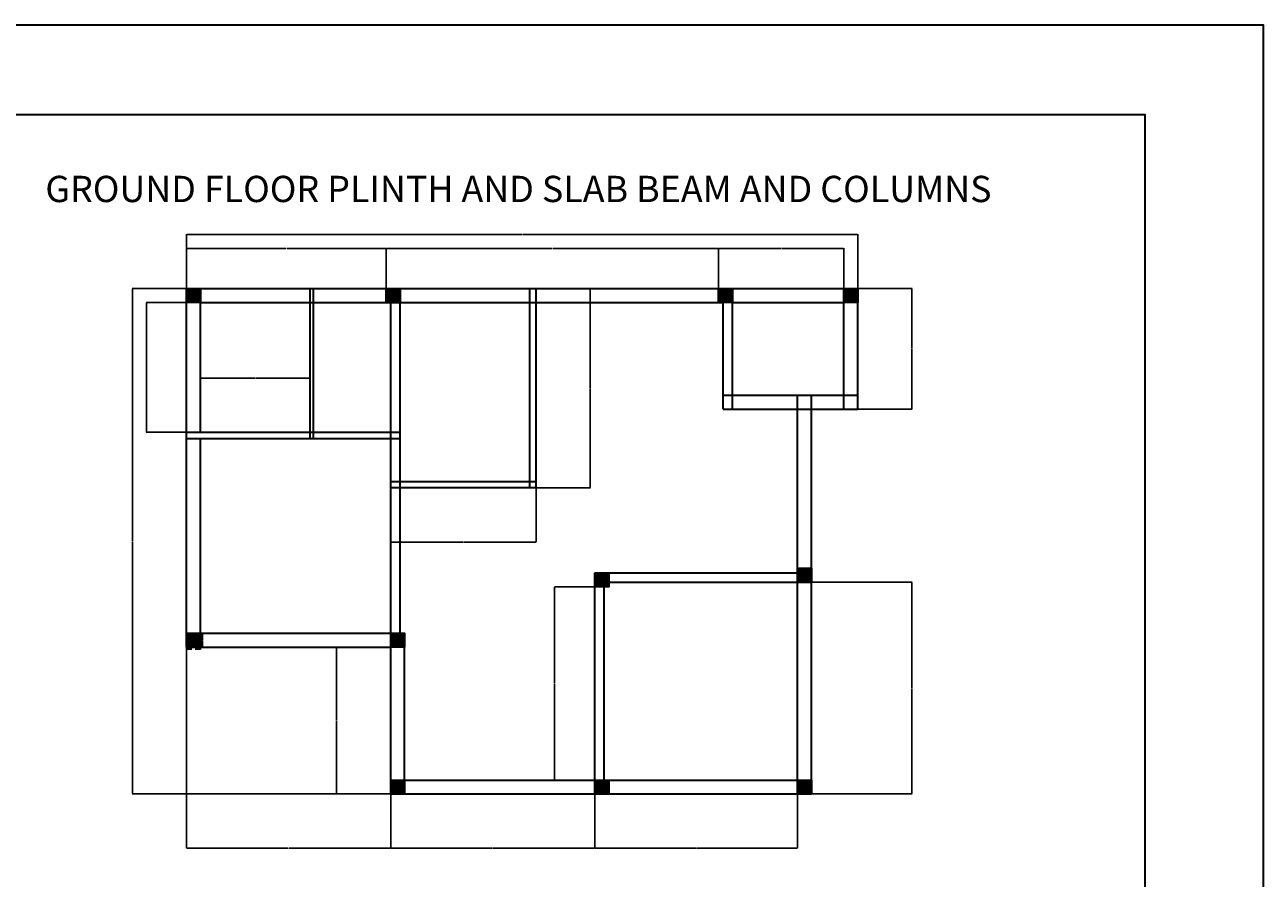
# Model space of a CAD drawing. Units: inches. Extents: x 2286 to 3750, y 1240 to 2345.
# Tile 7 of 7: x 2949 to 3750, y 1793 to 2345. Entities that reach past the tile are written whole.
import ezdxf

# ---------------------------------------------------------------- set-up
doc = ezdxf.new("R2010")
doc.units = ezdxf.units.IN
for name, color, linetype, lineweight in [('A-ANNO-DIMS', 2, 'Continuous', 18), ('A-ANNO-TEXT', 7, 'Continuous', 35), ('A-WALL', 7, 'Continuous', 35), ('S-BEAM', 7, 'Continuous', 30), ('S-COLS', 1, 'Continuous', 35)]:
    doc.layers.add(name, color=color, linetype=linetype, lineweight=lineweight)
doc.styles.get("Standard").update_dxf_attribs({"font": 'arial.ttf'})
doc.dimstyles.get("Standard").update_dxf_attribs({"dimtxt": 0.18, "dimasz": 0.18, "dimexe": 0.18, "dimexo": 0.0625, "dimgap": 0.09, "dimtad": 0, "dimtih": 1, "dimtoh": 1, "dimdec": 4, "dimzin": 0, "dimdsep": 46, "dimtxsty": 'Standard', "dimcen": 0.09, "dimadec": 0, "dimazin": 0, "dimtfac": 1, "dimtdec": 4, "dimtofl": 0, "dimtmove": 0, "dimatfit": 3, "dimfxl": 1, "dimtolj": 1, "dimtzin": 0, "dimarcsym": 0})

# ---------------------------------------------------------------- blocks, each defined once
blk = doc.blocks.new('COL-9-SQ')
h = blk.add_hatch(color=256)
h.dxf.hatch_style = 1
h.paths.add_polyline_path([(0, 0), (9, 0), (9, 9), (0, 9)])
blk.add_lwpolyline([(0, 9), (9, 9), (9, 0), (0, 0)], close=True)
blk = doc.blocks.new('*D22')
at = {"layer": 'A-ANNO-DIMS', "color": 0, "lineweight": -2, "transparency": 16777216}
for p, q in [((3054.05, 1942.13), (3054.05, 1940.66)), ((3054.23, 1940.84), (3057.51, 1940.84)), ((3062.87, 1940.84), (3059.59, 1940.84)), ((3063.05, 1942.13), (3063.05, 1940.66))]:
    blk.add_line(p, q, dxfattribs=at)
at = {"layer": 'A-ANNO-DIMS', "color": 0, "transparency": 16777216}
for points in [[(3054.23, 1940.87), (3054.23, 1940.81), (3054.05, 1940.84)], [(3062.87, 1940.87), (3062.87, 1940.81), (3063.05, 1940.84)]]:
    blk.add_solid(points, dxfattribs=at)
at = {"layer": 'Defpoints', "color": 0, "transparency": 16777216}
for p in [(3054.05, 1942.19), (3063.05, 1942.19), (3063.05, 1940.84)]:
    blk.add_point(p, dxfattribs=at)
at = {"layer": 'A-ANNO-DIMS', "color": 0, "transparency": 16777216, "insert": (3058.55, 1940.84), "char_height": 0.18, "attachment_point": 5}
blk.add_mtext('\\A1;COLUMN 9 TYP.', dxfattribs=at)
blk = doc.blocks.new('*D23')
at = {"layer": 'A-ANNO-DIMS', "color": 0, "lineweight": -2, "transparency": 16777216}
for p, q in [((3063.11, 1951.19), (3064.58, 1951.19)), ((3064.4, 1951.01), (3064.4, 1946.87)), ((3064.4, 1942.37), (3064.4, 1946.51)), ((3063.11, 1942.19), (3064.58, 1942.19))]:
    blk.add_line(p, q, dxfattribs=at)
at = {"layer": 'A-ANNO-DIMS', "color": 0, "transparency": 16777216}
for points in [[(3064.37, 1951.01), (3064.43, 1951.01), (3064.4, 1951.19)], [(3064.37, 1942.37), (3064.43, 1942.37), (3064.4, 1942.19)]]:
    blk.add_solid(points, dxfattribs=at)
at = {"layer": 'Defpoints', "color": 0, "transparency": 16777216}
for p in [(3063.05, 1951.19), (3064.4, 1951.19), (3063.05, 1942.19)]:
    blk.add_point(p, dxfattribs=at)
at = {"layer": 'A-ANNO-DIMS', "color": 0, "transparency": 16777216, "insert": (3064.4, 1946.69), "char_height": 0.18, "attachment_point": 5}
blk.add_mtext('\\A1;9 TYP.', dxfattribs=at)
blk = doc.blocks.new('*D93')
at = {"layer": 'A-ANNO-DIMS', "color": 0, "lineweight": -2, "transparency": 16777216}
for p, q in [((3054.05, 2174.25), (3054.05, 2209.37)), ((3054.23, 2209.19), (3270.76, 2209.19)), ((3487.87, 2209.19), (3271.34, 2209.19)), ((3488.05, 2174.25), (3488.05, 2209.37))]:
    blk.add_line(p, q, dxfattribs=at)
at = {"layer": 'A-ANNO-DIMS', "color": 0, "transparency": 16777216}
for points in [[(3054.23, 2209.22), (3054.23, 2209.16), (3054.05, 2209.19)], [(3487.87, 2209.22), (3487.87, 2209.16), (3488.05, 2209.19)]]:
    blk.add_solid(points, dxfattribs=at)
at = {"layer": 'Defpoints', "color": 0, "transparency": 16777216}
for p in [(3488.05, 2209.19), (3054.05, 2174.19), (3488.05, 2174.19)]:
    blk.add_point(p, dxfattribs=at)
at = {"layer": 'A-ANNO-DIMS', "color": 0, "transparency": 16777216, "insert": (3271.05, 2209.19), "char_height": 0.18, "attachment_point": 5}
blk.add_mtext('\\A1;434', dxfattribs=at)
blk = doc.blocks.new('*D94')
at = {"layer": 'A-ANNO-DIMS', "color": 0, "lineweight": -2, "transparency": 16777216}
for p, q in [((3053.99, 2174.19), (3018.87, 2174.19)), ((3019.05, 2174.01), (3019.05, 2010.87)), ((3019.05, 1847.37), (3019.05, 2010.51)), ((3185.99, 1847.19), (3018.87, 1847.19))]:
    blk.add_line(p, q, dxfattribs=at)
at = {"layer": 'A-ANNO-DIMS', "color": 0, "transparency": 16777216}
for points in [[(3019.02, 2174.01), (3019.08, 2174.01), (3019.05, 2174.19)], [(3019.02, 1847.37), (3019.08, 1847.37), (3019.05, 1847.19)]]:
    blk.add_solid(points, dxfattribs=at)
at = {"layer": 'Defpoints', "color": 0, "transparency": 16777216}
for p in [(3054.05, 2174.19), (3019.05, 1847.19), (3186.05, 1847.19)]:
    blk.add_point(p, dxfattribs=at)
at = {"layer": 'A-ANNO-DIMS', "color": 0, "transparency": 16777216, "insert": (3019.05, 2010.69), "char_height": 0.18, "attachment_point": 5}
blk.add_mtext('\\A1;327', dxfattribs=at)
blk = doc.blocks.new('*D95')
at = {"layer": 'A-ANNO-DIMS', "color": 0, "lineweight": -2, "transparency": 16777216}
for p, q in [((3054.05, 2165.25), (3054.05, 2200.37)), ((3054.23, 2200.19), (3118.27, 2200.19)), ((3182.87, 2200.19), (3118.83, 2200.19)), ((3183.05, 2165.25), (3183.05, 2200.37))]:
    blk.add_line(p, q, dxfattribs=at)
at = {"layer": 'A-ANNO-DIMS', "color": 0, "transparency": 16777216}
for points in [[(3054.23, 2200.22), (3054.23, 2200.16), (3054.05, 2200.19)], [(3182.87, 2200.22), (3182.87, 2200.16), (3183.05, 2200.19)]]:
    blk.add_solid(points, dxfattribs=at)
at = {"layer": 'Defpoints', "color": 0, "transparency": 16777216}
for p in [(3183.05, 2200.19), (3054.05, 2165.19), (3183.05, 2165.19)]:
    blk.add_point(p, dxfattribs=at)
at = {"layer": 'A-ANNO-DIMS', "color": 0, "transparency": 16777216, "insert": (3118.55, 2200.19), "char_height": 0.18, "attachment_point": 5}
blk.add_mtext('\\A1;129', dxfattribs=at)
blk = doc.blocks.new('*D96')
at = {"layer": 'A-ANNO-DIMS', "color": 0, "lineweight": -2, "transparency": 16777216}
for p, q in [((3183.05, 2165.25), (3183.05, 2200.37)), ((3183.23, 2200.19), (3290.26, 2200.19)), ((3397.87, 2200.19), (3290.84, 2200.19)), ((3398.05, 2165.25), (3398.05, 2200.37))]:
    blk.add_line(p, q, dxfattribs=at)
at = {"layer": 'A-ANNO-DIMS', "color": 0, "transparency": 16777216}
for points in [[(3183.23, 2200.22), (3183.23, 2200.16), (3183.05, 2200.19)], [(3397.87, 2200.22), (3397.87, 2200.16), (3398.05, 2200.19)]]:
    blk.add_solid(points, dxfattribs=at)
at = {"layer": 'Defpoints', "color": 0, "transparency": 16777216}
for p in [(3398.05, 2200.19), (3183.05, 2165.19), (3398.05, 2165.19)]:
    blk.add_point(p, dxfattribs=at)
at = {"layer": 'A-ANNO-DIMS', "color": 0, "transparency": 16777216, "insert": (3290.55, 2200.19), "char_height": 0.18, "attachment_point": 5}
blk.add_mtext('\\A1;215', dxfattribs=at)
blk = doc.blocks.new('*D97')
at = {"layer": 'A-ANNO-DIMS', "color": 0, "lineweight": -2, "transparency": 16777216}
for p, q in [((3398.05, 2165.25), (3398.05, 2200.37)), ((3398.23, 2200.19), (3438.35, 2200.19)), ((3478.87, 2200.19), (3438.75, 2200.19)), ((3479.05, 2165.25), (3479.05, 2200.37))]:
    blk.add_line(p, q, dxfattribs=at)
at = {"layer": 'A-ANNO-DIMS', "color": 0, "transparency": 16777216}
for points in [[(3398.23, 2200.22), (3398.23, 2200.16), (3398.05, 2200.19)], [(3478.87, 2200.22), (3478.87, 2200.16), (3479.05, 2200.19)]]:
    blk.add_solid(points, dxfattribs=at)
at = {"layer": 'Defpoints', "color": 0, "transparency": 16777216}
for p in [(3479.05, 2200.19), (3398.05, 2165.19), (3479.05, 2165.19)]:
    blk.add_point(p, dxfattribs=at)
at = {"layer": 'A-ANNO-DIMS', "color": 0, "transparency": 16777216, "insert": (3438.55, 2200.19), "char_height": 0.18, "attachment_point": 5}
blk.add_mtext('\\A1;81', dxfattribs=at)
blk = doc.blocks.new('*D98')
at = {"layer": 'A-ANNO-DIMS', "color": 0, "lineweight": -2, "transparency": 16777216}
for p, q in [((3054.05, 1942.13), (3054.05, 1812.01)), ((3186.05, 1942.13), (3186.05, 1812.01)), ((3054.23, 1812.19), (3119.77, 1812.19)), ((3185.87, 1812.19), (3120.33, 1812.19))]:
    blk.add_line(p, q, dxfattribs=at)
at = {"layer": 'A-ANNO-DIMS', "color": 0, "transparency": 16777216}
for points in [[(3054.23, 1812.22), (3054.23, 1812.16), (3054.05, 1812.19)], [(3185.87, 1812.22), (3185.87, 1812.16), (3186.05, 1812.19)]]:
    blk.add_solid(points, dxfattribs=at)
at = {"layer": 'Defpoints', "color": 0, "transparency": 16777216}
for p in [(3054.05, 1942.19), (3186.05, 1942.19), (3186.05, 1812.19)]:
    blk.add_point(p, dxfattribs=at)
at = {"layer": 'A-ANNO-DIMS', "color": 0, "transparency": 16777216, "insert": (3120.05, 1812.19), "char_height": 0.18, "attachment_point": 5}
blk.add_mtext('\\A1;132', dxfattribs=at)
blk = doc.blocks.new('*D99')
at = {"layer": 'A-ANNO-DIMS', "color": 0, "lineweight": -2, "transparency": 16777216}
for p, q in [((3186.05, 1847.13), (3186.05, 1812.01)), ((3318.05, 1847.13), (3318.05, 1812.01)), ((3186.23, 1812.19), (3251.77, 1812.19)), ((3317.87, 1812.19), (3252.33, 1812.19))]:
    blk.add_line(p, q, dxfattribs=at)
at = {"layer": 'A-ANNO-DIMS', "color": 0, "transparency": 16777216}
for points in [[(3186.23, 1812.22), (3186.23, 1812.16), (3186.05, 1812.19)], [(3317.87, 1812.22), (3317.87, 1812.16), (3318.05, 1812.19)]]:
    blk.add_solid(points, dxfattribs=at)
at = {"layer": 'Defpoints', "color": 0, "transparency": 16777216}
for p in [(3186.05, 1847.19), (3318.05, 1847.19), (3318.05, 1812.19)]:
    blk.add_point(p, dxfattribs=at)
at = {"layer": 'A-ANNO-DIMS', "color": 0, "transparency": 16777216, "insert": (3252.05, 1812.19), "char_height": 0.18, "attachment_point": 5}
blk.add_mtext('\\A1;132', dxfattribs=at)
blk = doc.blocks.new('*D100')
at = {"layer": 'A-ANNO-DIMS', "color": 0, "lineweight": -2, "transparency": 16777216}
for p, q in [((3318.05, 1847.13), (3318.05, 1812.01)), ((3449.05, 1847.13), (3449.05, 1812.01)), ((3318.23, 1812.19), (3383.29, 1812.19)), ((3448.87, 1812.19), (3383.81, 1812.19))]:
    blk.add_line(p, q, dxfattribs=at)
at = {"layer": 'A-ANNO-DIMS', "color": 0, "transparency": 16777216}
for points in [[(3318.23, 1812.22), (3318.23, 1812.16), (3318.05, 1812.19)], [(3448.87, 1812.22), (3448.87, 1812.16), (3449.05, 1812.19)]]:
    blk.add_solid(points, dxfattribs=at)
at = {"layer": 'Defpoints', "color": 0, "transparency": 16777216}
for p in [(3318.05, 1847.19), (3449.05, 1847.19), (3449.05, 1812.19)]:
    blk.add_point(p, dxfattribs=at)
at = {"layer": 'A-ANNO-DIMS', "color": 0, "transparency": 16777216, "insert": (3383.55, 1812.19), "char_height": 0.18, "attachment_point": 5}
blk.add_mtext('\\A1;131', dxfattribs=at)
blk = doc.blocks.new('*D101')
at = {"layer": 'A-ANNO-DIMS', "color": 0, "lineweight": -2, "transparency": 16777216}
for p, q in [((3185.99, 1942.19), (3150.87, 1942.19)), ((3151.05, 1942.01), (3151.05, 1894.87)), ((3151.05, 1847.37), (3151.05, 1894.51)), ((3185.99, 1847.19), (3150.87, 1847.19))]:
    blk.add_line(p, q, dxfattribs=at)
at = {"layer": 'A-ANNO-DIMS', "color": 0, "transparency": 16777216}
for points in [[(3151.02, 1942.01), (3151.08, 1942.01), (3151.05, 1942.19)], [(3151.02, 1847.37), (3151.08, 1847.37), (3151.05, 1847.19)]]:
    blk.add_solid(points, dxfattribs=at)
at = {"layer": 'Defpoints', "color": 0, "transparency": 16777216}
for p in [(3151.05, 1942.19), (3186.05, 1942.19), (3186.05, 1847.19)]:
    blk.add_point(p, dxfattribs=at)
at = {"layer": 'A-ANNO-DIMS', "color": 0, "transparency": 16777216, "insert": (3151.05, 1894.69), "char_height": 0.18, "attachment_point": 5}
blk.add_mtext('\\A1;95', dxfattribs=at)
blk = doc.blocks.new('*D102')
at = {"layer": 'A-ANNO-DIMS', "color": 0, "lineweight": -2, "transparency": 16777216}
for p, q in [((3458.11, 1984.19), (3523.23, 1984.19)), ((3523.05, 1984.01), (3523.05, 1915.87)), ((3523.05, 1847.37), (3523.05, 1915.51)), ((3458.11, 1847.19), (3523.23, 1847.19))]:
    blk.add_line(p, q, dxfattribs=at)
at = {"layer": 'A-ANNO-DIMS', "color": 0, "transparency": 16777216}
for points in [[(3523.02, 1984.01), (3523.08, 1984.01), (3523.05, 1984.19)], [(3523.02, 1847.37), (3523.08, 1847.37), (3523.05, 1847.19)]]:
    blk.add_solid(points, dxfattribs=at)
at = {"layer": 'Defpoints', "color": 0, "transparency": 16777216}
for p in [(3458.05, 1984.19), (3523.05, 1984.19), (3458.05, 1847.19)]:
    blk.add_point(p, dxfattribs=at)
at = {"layer": 'A-ANNO-DIMS', "color": 0, "transparency": 16777216, "insert": (3523.05, 1915.69), "char_height": 0.18, "attachment_point": 5}
blk.add_mtext('\\A1;137', dxfattribs=at)
blk = doc.blocks.new('*D103')
at = {"layer": 'A-ANNO-DIMS', "color": 0, "lineweight": -2, "transparency": 16777216}
for p, q in [((3488.11, 2174.19), (3523.23, 2174.19)), ((3523.05, 2174.01), (3523.05, 2135.37)), ((3523.05, 2096.37), (3523.05, 2135.01)), ((3488.11, 2096.19), (3523.23, 2096.19))]:
    blk.add_line(p, q, dxfattribs=at)
at = {"layer": 'A-ANNO-DIMS', "color": 0, "transparency": 16777216}
for points in [[(3523.02, 2174.01), (3523.08, 2174.01), (3523.05, 2174.19)], [(3523.02, 2096.37), (3523.08, 2096.37), (3523.05, 2096.19)]]:
    blk.add_solid(points, dxfattribs=at)
at = {"layer": 'Defpoints', "color": 0, "transparency": 16777216}
for p in [(3488.05, 2174.19), (3523.05, 2174.19), (3488.05, 2096.19)]:
    blk.add_point(p, dxfattribs=at)
at = {"layer": 'A-ANNO-DIMS', "color": 0, "transparency": 16777216, "insert": (3523.05, 2135.19), "char_height": 0.18, "attachment_point": 5}
blk.add_mtext('\\A1;78', dxfattribs=at)
blk = doc.blocks.new('*D104')
at = {"layer": 'A-ANNO-DIMS', "color": 0, "lineweight": -2, "transparency": 16777216}
for p, q in [((3063.05, 2081.25), (3063.05, 2116.37)), ((3063.23, 2116.19), (3098.35, 2116.19)), ((3133.87, 2116.19), (3098.75, 2116.19)), ((3134.05, 2081.25), (3134.05, 2116.37))]:
    blk.add_line(p, q, dxfattribs=at)
at = {"layer": 'A-ANNO-DIMS', "color": 0, "transparency": 16777216}
for points in [[(3063.23, 2116.22), (3063.23, 2116.16), (3063.05, 2116.19)], [(3133.87, 2116.22), (3133.87, 2116.16), (3134.05, 2116.19)]]:
    blk.add_solid(points, dxfattribs=at)
at = {"layer": 'Defpoints', "color": 0, "transparency": 16777216}
for p in [(3134.05, 2116.19), (3063.05, 2081.19), (3134.05, 2081.19)]:
    blk.add_point(p, dxfattribs=at)
at = {"layer": 'A-ANNO-DIMS', "color": 0, "transparency": 16777216, "insert": (3098.55, 2116.19), "char_height": 0.18, "attachment_point": 5}
blk.add_mtext('\\A1;71', dxfattribs=at)
blk = doc.blocks.new('*D105')
at = {"layer": 'A-ANNO-DIMS', "color": 0, "lineweight": -2, "transparency": 16777216}
for p, q in [((3062.99, 2165.19), (3027.87, 2165.19)), ((3028.05, 2165.01), (3028.05, 2123.37)), ((3028.05, 2081.37), (3028.05, 2123.01)), ((3062.99, 2081.19), (3027.87, 2081.19))]:
    blk.add_line(p, q, dxfattribs=at)
at = {"layer": 'A-ANNO-DIMS', "color": 0, "transparency": 16777216}
for points in [[(3028.02, 2165.01), (3028.08, 2165.01), (3028.05, 2165.19)], [(3028.02, 2081.37), (3028.08, 2081.37), (3028.05, 2081.19)]]:
    blk.add_solid(points, dxfattribs=at)
at = {"layer": 'Defpoints', "color": 0, "transparency": 16777216}
for p in [(3028.05, 2165.19), (3063.05, 2165.19), (3063.05, 2081.19)]:
    blk.add_point(p, dxfattribs=at)
at = {"layer": 'A-ANNO-DIMS', "color": 0, "transparency": 16777216, "insert": (3028.05, 2123.19), "char_height": 0.18, "attachment_point": 5}
blk.add_mtext('\\A1;84', dxfattribs=at)
blk = doc.blocks.new('*D106')
at = {"layer": 'A-ANNO-DIMS', "color": 0, "lineweight": -2, "transparency": 16777216}
for p, q in [((3186.05, 2045.13), (3186.05, 2010.01)), ((3280.05, 2045.13), (3280.05, 2010.01)), ((3186.23, 2010.19), (3232.83, 2010.19)), ((3279.87, 2010.19), (3233.27, 2010.19))]:
    blk.add_line(p, q, dxfattribs=at)
at = {"layer": 'A-ANNO-DIMS', "color": 0, "transparency": 16777216}
for points in [[(3186.23, 2010.22), (3186.23, 2010.16), (3186.05, 2010.19)], [(3279.87, 2010.22), (3279.87, 2010.16), (3280.05, 2010.19)]]:
    blk.add_solid(points, dxfattribs=at)
at = {"layer": 'Defpoints', "color": 0, "transparency": 16777216}
for p in [(3186.05, 2045.19), (3280.05, 2045.19), (3186.05, 2010.19)]:
    blk.add_point(p, dxfattribs=at)
at = {"layer": 'A-ANNO-DIMS', "color": 0, "transparency": 16777216, "insert": (3233.05, 2010.19), "char_height": 0.18, "attachment_point": 5}
blk.add_mtext('\\A1;94', dxfattribs=at)
blk = doc.blocks.new('*D107')
at = {"layer": 'A-ANNO-DIMS', "color": 0, "lineweight": -2, "transparency": 16777216}
for p, q in [((3280.11, 2174.19), (3315.23, 2174.19)), ((3315.05, 2174.01), (3315.05, 2109.87)), ((3315.05, 2045.37), (3315.05, 2109.51)), ((3280.11, 2045.19), (3315.23, 2045.19))]:
    blk.add_line(p, q, dxfattribs=at)
at = {"layer": 'A-ANNO-DIMS', "color": 0, "transparency": 16777216}
for points in [[(3315.02, 2174.01), (3315.08, 2174.01), (3315.05, 2174.19)], [(3315.02, 2045.37), (3315.08, 2045.37), (3315.05, 2045.19)]]:
    blk.add_solid(points, dxfattribs=at)
at = {"layer": 'Defpoints', "color": 0, "transparency": 16777216}
for p in [(3280.05, 2174.19), (3280.05, 2045.19), (3315.05, 2045.19)]:
    blk.add_point(p, dxfattribs=at)
at = {"layer": 'A-ANNO-DIMS', "color": 0, "transparency": 16777216, "insert": (3315.05, 2109.69), "char_height": 0.18, "attachment_point": 5}
blk.add_mtext('\\A1;129', dxfattribs=at)
blk = doc.blocks.new('*D108')
at = {"layer": 'A-ANNO-DIMS', "color": 0, "lineweight": -2, "transparency": 16777216}
for p, q in [((3326.99, 1981.19), (3291.87, 1981.19)), ((3292.05, 1981.01), (3292.05, 1918.87)), ((3292.05, 1856.37), (3292.05, 1918.51)), ((3326.99, 1856.19), (3291.87, 1856.19))]:
    blk.add_line(p, q, dxfattribs=at)
at = {"layer": 'A-ANNO-DIMS', "color": 0, "transparency": 16777216}
for points in [[(3292.02, 1981.01), (3292.08, 1981.01), (3292.05, 1981.19)], [(3292.02, 1856.37), (3292.08, 1856.37), (3292.05, 1856.19)]]:
    blk.add_solid(points, dxfattribs=at)
at = {"layer": 'Defpoints', "color": 0, "transparency": 16777216}
for p in [(3292.05, 1981.19), (3327.05, 1981.19), (3327.05, 1856.19)]:
    blk.add_point(p, dxfattribs=at)
at = {"layer": 'A-ANNO-DIMS', "color": 0, "transparency": 16777216, "insert": (3292.05, 1918.69), "char_height": 0.18, "attachment_point": 5}
blk.add_mtext('\\A1;125', dxfattribs=at)

msp = doc.modelspace()

# ---------------------------------------------------------------- linework, layer by layer
at = {"layer": 'A-WALL'}
for points in [[(2286.2079, 2344.8717), (3750.2574, 2344.8717), (3750.2574, 1240.4105), (2286.2079, 1240.4105)], [(2354.794, 2286.8809), (3673.7575, 2286.8809), (3673.7575, 1335.3046), (2354.794, 1335.3046)]]:
    msp.add_lwpolyline(points, close=True, dxfattribs=at)
at = {"layer": 'S-BEAM'}
for p, q in [((3054.0502, 2174.1892), (3488.0502, 2174.1892)), ((3054.0502, 1942.1892), (3054.0502, 2174.1892)), ((3134.0502, 2077.1892), (3134.0502, 2174.1892)), ((3136.0502, 2077.1892), (3136.0502, 2174.1892)), ((3276.0502, 2045.1892), (3276.0502, 2174.1892)), ((3280.0502, 2045.1892), (3280.0502, 2174.1892)), ((3488.0502, 2096.1892), (3488.0502, 2174.1892)), ((3063.0502, 2165.1892), (3401.0502, 2165.1892)), ((3063.0502, 2081.1892), (3063.0502, 2165.1892)), ((3186.0502, 2077.1892), (3186.0502, 2165.1892)), ((3192.0502, 1951.1892), (3192.0502, 2165.1892)), ((3401.0502, 2096.1892), (3401.0502, 2165.1892)), ((3407.0502, 2165.1892), (3479.0502, 2165.1892)), ((3407.0502, 2096.1892), (3407.0502, 2165.1892)), ((3479.0502, 2096.1892), (3479.0502, 2165.1892)), ((3401.0502, 2105.1892), (3488.0502, 2105.1892)), ((3449.0502, 1993.1892), (3449.0502, 2105.1892)), ((3458.0502, 1993.1892), (3458.0502, 2105.1892)), ((3401.0502, 2096.1892), (3488.0502, 2096.1892)), ((3443.0502, 2096.1892), (3449.0502, 2096.1892)), ((3134.0502, 2077.1892), (3134.0502, 2083.1892)), ((3054.0502, 2081.1892), (3186.0502, 2081.1892)), ((3054.0502, 2077.1892), (3186.0502, 2077.1892)), ((3063.0502, 2081.1892), (3134.0502, 2081.1892)), ((3063.0502, 1942.1892), (3063.0502, 2077.1892)), ((3136.0502, 2077.1892), (3192.0502, 2077.1892)), ((3162.0502, 2081.1892), (3192.0502, 2081.1892)), ((3186.0502, 1942.1892), (3186.0502, 2077.1892)), ((3280.0502, 2049.1892), (3186.0502, 2049.1892)), ((3280.0502, 2045.1892), (3186.0502, 2045.1892)), ((3449.0502, 1990.1892), (3449.0502, 2019.1892)), ((3458.0502, 1847.1892), (3458.0502, 2019.1892)), ((3318.0502, 1990.1892), (3449.0502, 1990.1892)), ((3318.0502, 1856.1892), (3318.0502, 1990.1892)), ((3401.0502, 1990.1892), (3449.0502, 1990.1892)), ((3324.0502, 1984.1892), (3449.0502, 1984.1892)), ((3324.0502, 1856.1892), (3324.0502, 1984.1892)), ((3401.0502, 1984.1892), (3449.0502, 1984.1892)), ((3449.0502, 1984.1892), (3458.0502, 1984.1892)), ((3449.0502, 1847.1892), (3449.0502, 1984.1892)), ((3054.0502, 1951.1892), (3186.0502, 1951.1892)), ((3186.0502, 1951.1892), (3186.0502, 1953.1892)), ((3195.0502, 1847.1892), (3195.0502, 1951.1892)), ((3054.0502, 1942.1892), (3186.0502, 1942.1892)), ((3186.0502, 1847.1892), (3186.0502, 1942.1892)), ((3186.0502, 1856.1892), (3318.0502, 1856.1892)), ((3324.0502, 1856.1892), (3458.0502, 1856.1892)), ((3186.0502, 1847.1892), (3458.0502, 1847.1892))]:
    msp.add_line(p, q, dxfattribs=at)

# ---------------------------------------------------------------- block references
at = {"layer": 'S-COLS'}
for p in [(3054.0502, 2165.1892), (3183.0502, 2165.1892), (3398.0502, 2165.1892), (3479.0502, 2165.1892), (3318.0502, 1981.1892), (3449.0502, 1984.1892), (3054.0502, 1942.1892), (3186.0502, 1942.1892), (3186.0502, 1847.1892), (3318.0502, 1847.1892), (3449.0502, 1847.1892)]:
    msp.add_blockref('COL-9-SQ', p, dxfattribs=at)

# ---------------------------------------------------------------- texts
at = {"layer": 'A-ANNO-TEXT'}
msp.add_text('GROUND FLOOR PLINTH AND SLAB BEAM AND COLUMNS', height=17, dxfattribs=at).set_placement((2962.6875, 2230.1297))

# ---------------------------------------------------------------- dimensions: what is measured, and where the dimension line sits
at = {"layer": 'A-ANNO-DIMS'}
for base, p1, p2, picture, middle in [((3488.0502, 2209.1892), (3054.0502, 2174.1892), (3488.0502, 2174.1892), '*D93', (3271.0502, 2209.1892)), ((3183.0502, 2200.1892), (3054.0502, 2165.1892), (3183.0502, 2165.1892), '*D95', (3118.5502, 2200.1892)), ((3398.0502, 2200.1892), (3183.0502, 2165.1892), (3398.0502, 2165.1892), '*D96', (3290.5502, 2200.1892)), ((3134.0502, 2116.1892), (3063.0502, 2081.1892), (3134.0502, 2081.1892), '*D104', (3098.5502, 2116.1892)), ((3186.0502, 1812.1892), (3054.0502, 1942.1892), (3186.0502, 1942.1892), '*D98', (3120.0502, 1812.1892)), ((3318.0502, 1812.1892), (3186.0502, 1847.1892), (3318.0502, 1847.1892), '*D99', (3252.0502, 1812.1892)), ((3449.0502, 1812.1892), (3318.0502, 1847.1892), (3449.0502, 1847.1892), '*D100', (3383.5502, 1812.1892))]:
    dim = msp.add_linear_dim(base=base, p1=p1, p2=p2, dimstyle='Standard', override={"dimdec": 0, "dimlfac": 1, "dimrnd": 0, "dimzin": 0, "dimdsep": 46, "dimlunit": 2}, dxfattribs=at)
    dim.commit()
    dim.dimension.update_dxf_attribs({"geometry": picture, "text_midpoint": middle})
for base, p1, p2, angle, picture, middle in [((3479.0502, 2200.1892), (3398.0502, 2165.1892), (3479.0502, 2165.1892), 0, '*D97', (3438.5502, 2200.1892)), ((3019.0503, 1847.1892), (3054.0502, 2174.1892), (3186.0502, 1847.1892), 90, '*D94', (3019.0503, 2010.6892)), ((3315.0503, 2045.1892), (3280.0502, 2174.1892), (3280.0502, 2045.1892), 270, '*D107', (3315.0503, 2109.6892)), ((3523.0503, 2174.1892), (3488.0502, 2096.1892), (3488.0502, 2174.1892), 90, '*D103', (3523.0503, 2135.1892)), ((3028.0503, 2165.1892), (3063.0502, 2081.1892), (3063.0502, 2165.1892), 90, '*D105', (3028.0503, 2123.1892)), ((3186.0502, 2010.1892), (3280.0502, 2045.1892), (3186.0502, 2045.1892), 180, '*D106', (3233.0502, 2010.1892)), ((3292.0503, 1981.1892), (3327.0502, 1856.1892), (3327.0502, 1981.1892), 90, '*D108', (3292.0503, 1918.6892)), ((3523.0503, 1984.1892), (3458.0502, 1847.1892), (3458.0502, 1984.1892), 90, '*D102', (3523.0503, 1915.6892)), ((3151.0503, 1942.1892), (3186.0502, 1847.1892), (3186.0502, 1942.1892), 90, '*D101', (3151.0503, 1894.6892))]:
    dim = msp.add_linear_dim(base=base, p1=p1, p2=p2, angle=angle, dimstyle='Standard', override={"dimdec": 0, "dimlfac": 1, "dimrnd": 0, "dimzin": 0, "dimdsep": 46, "dimlunit": 2}, dxfattribs=at)
    dim.commit()
    dim.dimension.update_dxf_attribs({"geometry": picture, "text_midpoint": middle})
dim = msp.add_linear_dim(base=(3064.4002, 1951.1892), p1=(3063.0502, 1942.1892), p2=(3063.0502, 1951.1892), angle=90, text='<> TYP.', dimstyle='Standard', override={"dimdec": 0, "dimlfac": 1, "dimrnd": 0, "dimzin": 0, "dimdsep": 46, "dimlunit": 2}, dxfattribs=at)
dim.commit()
dim.dimension.update_dxf_attribs({"geometry": '*D23', "text_midpoint": (3064.4002, 1946.6892)})
dim = msp.add_linear_dim(base=(3063.0502, 1940.8392), p1=(3054.0502, 1942.1892), p2=(3063.0502, 1942.1892), text='COLUMN <> TYP.', dimstyle='Standard', override={"dimdec": 0, "dimlfac": 1, "dimrnd": 0, "dimzin": 0, "dimdsep": 46, "dimlunit": 2}, dxfattribs=at)
dim.commit()
dim.dimension.update_dxf_attribs({"geometry": '*D22', "text_midpoint": (3058.5502, 1940.8392)})

doc.saveas('drawing.dxf')
